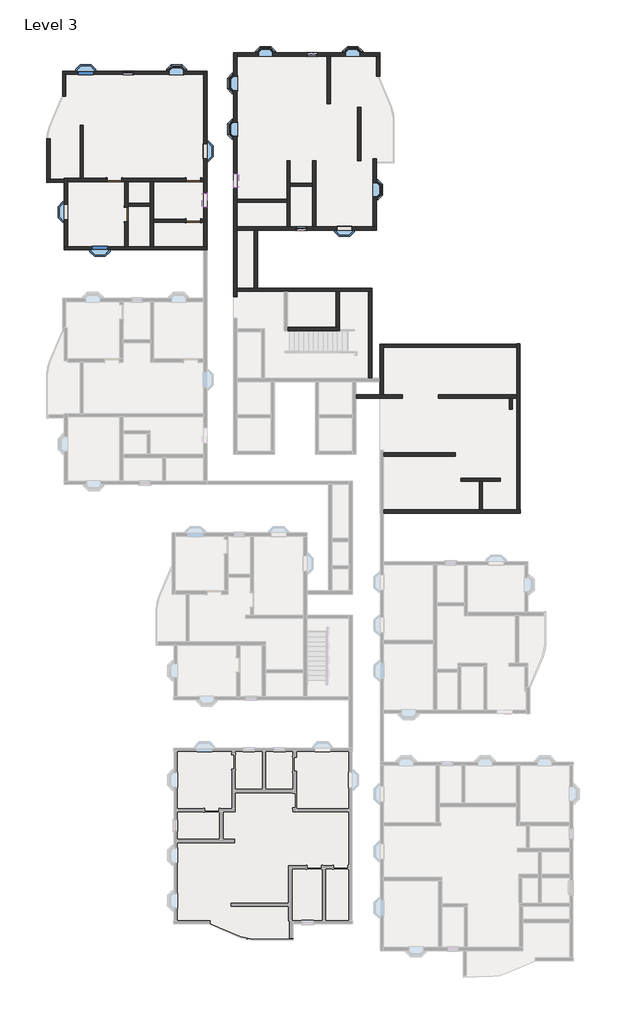
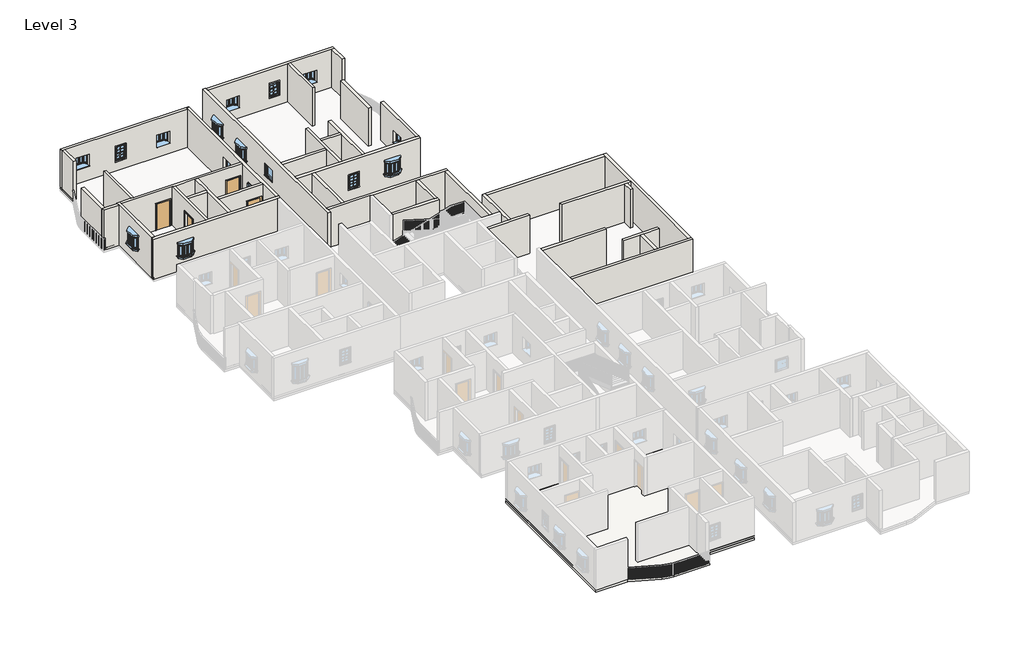
# One storey, part 4 of 14: 39 walls, 16 windows, 4 doors, 1 roof, 1 slab.
"""IFC4 building model written with IfcOpenShell, lengths in millimetres."""

from ifc_helpers import new_model, si_unit, point, frame, frame_2d, origin, place, context, project, spatial, polyline, circle_curve, trimmed, segment, composite_curve, outline, extrude, faceted_brep, transform, mapped, element, save
from components import door_719f80de, window_910x910mm_67ef725a, window_8debb0fa, windows_sgl_w_glazing_bars_910x910mm_256712d0

model = new_model("IFC4")

# Units and contexts
model_context = context("Model", 3, world=origin())
ifc_project = project(units=[si_unit("LENGTHUNIT", "METRE", prefix="MILLI")], contexts=[model_context])

# Site, building, storey
site = spatial("IfcSite", under=ifc_project)
building = spatial("IfcBuilding", under=site)
storey = spatial("IfcBuildingStorey", under=building, Name="Level 3", Elevation=6096.0)

# Doors
placement = place(None, origin())
door_shape = door_719f80de(model_context)
element("IfcDoor", 1, ObjectType="Single-Flush : 36\" x 84\"", at=placement, inside=storey, context=model_context, shape_type="MappedRepresentation", body=[
    mapped(door_shape, transform((-16068.1391351, 22048.4083494, 6096.0), x_axis=(1.0, 0.0, 0.0), y_axis=(0.0, 1.0, 0.0), z_axis=(0.0, 0.0, 1.0))),
])
element("IfcDoor", 2, ObjectType="Single-Flush : 36\" x 84\"", at=placement, inside=storey, context=model_context, shape_type="MappedRepresentation", body=[
    mapped(door_shape, transform((-15306.1391351, 19864.0083494, 6096.0), x_axis=(0.0, 1.0, 0.0), y_axis=(-1.0, 0.0, 0.0), z_axis=(0.0, 0.0, 1.0))),
])
element("IfcDoor", 3, ObjectType="Single-Flush : 36\" x 84\"", at=placement, inside=storey, context=model_context, shape_type="MappedRepresentation", body=[
    mapped(door_shape, transform((-11057.9891351, 19470.3083494, 6096.0), x_axis=(1.0, 0.0, 0.0), y_axis=(0.0, 1.0, 0.0), z_axis=(0.0, 0.0, 1.0))),
])
element("IfcDoor", 4, ObjectType="Single-Flush : 36\" x 84\"", at=placement, inside=storey, context=model_context, shape_type="MappedRepresentation", body=[
    mapped(door_shape, transform((-11057.9891351, 22048.4083494, 6096.0), x_axis=(1.0, 0.0, 0.0), y_axis=(0.0, 1.0, 0.0), z_axis=(0.0, 0.0, 1.0))),
])

# Roof
element("IfcRoof", 5, ObjectType="Generic - 12\"", at=placement, inside=storey, context=model_context, shape_type="SweptSolid", body=[
    extrude(outline(composite_curve([segment(polyline([(-10024.8708389, -25100.3416506), (-12290.487215, -25100.3416506), (-12290.487215, -13962.4416506), (-986.8891351, -13962.4416506), (-986.8891351, -25100.3416506), (-4746.0891351, -25100.3416506), (-4746.0891351, -26090.9416506), (-7315.6413127, -26090.9416506)]), True, "CONTINUOUS"), segment(trimmed(circle_curve(frame_2d((-7315.6413127, -24160.5416506)), 1930.4), [point((-7315.6413127, -26090.9416506))], [point((-8075.5356374, -25935.0851906))], False, "CARTESIAN"), True, "CONTINUOUS"), segment(polyline([(-8075.5356374, -25935.0851906), (-10024.8708389, -25100.3416506)]), True, "CONTINUOUS")], self_intersect=False)), frame((0.0, 0.0, 6096.0), z_axis=(0.0, 0.0, 1.0), x_axis=(1.0, 0.0, 0.0)), (0.0, 0.0, 1.0), 152.4),
])

# Slab
element("IfcSlab", 6, ObjectType="Generic - 12\"", at=placement, inside=storey, context=model_context, shape_type="SweptSolid", body=[
    extrude(outline(composite_curve([segment(polyline([(-10024.8708389, -25100.3416506), (-12290.487215, -25100.3416506), (-12290.487215, -13962.4416506), (-986.8891351, -13962.4416506), (-986.8891351, -25100.3416506), (-4746.0891351, -25100.3416506), (-4746.0891351, -26090.9416506), (-7315.6413127, -26090.9416506)]), True, "CONTINUOUS"), segment(trimmed(circle_curve(frame_2d((-7315.6413127, -24160.5416506)), 1930.4), [point((-7315.6413127, -26090.9416506))], [point((-8075.5356374, -25935.0851906))], False, "CARTESIAN"), True, "CONTINUOUS"), segment(polyline([(-8075.5356374, -25935.0851906), (-10024.8708389, -25100.3416506)]), True, "CONTINUOUS")], self_intersect=False)), frame((0.0, 0.0, 5943.6), z_axis=(0.0, 0.0, 1.0), x_axis=(1.0, 0.0, 0.0)), (0.0, 0.0, 1.0), 152.4),
])

# Walls
element("IfcWall", 7, ObjectType="4.5\" p", at=placement, inside=storey, context=model_context, shape_type="Brep", body=[
    faceted_brep([(-10600.7891351, 21946.8083494, 8229.6), (-10600.7891351, 21946.8083494, 6096.0), (-10397.5891351, 21946.8083494, 6096.0), (-10397.5891351, 21946.8083494, 9144.0), (-13578.9391351, 21946.8083494, 9144.0), (-13782.1391351, 21946.8083494, 9144.0), (-15204.5391351, 21946.8083494, 9144.0), (-15407.7391351, 21946.8083494, 9144.0), (-19033.5891351, 21946.8083494, 9144.0), (-19033.5891351, 21946.8083494, 6096.0), (-16525.3391351, 21946.8083494, 6096.0), (-16525.3391351, 21946.8083494, 8229.6), (-15610.9391351, 21946.8083494, 8229.6), (-15610.9391351, 21946.8083494, 6096.0), (-15407.7391351, 21946.8083494, 6096.0), (-15204.5391351, 21946.8083494, 6096.0), (-13782.1391351, 21946.8083494, 6096.0), (-13578.9391351, 21946.8083494, 6096.0), (-11515.1891351, 21946.8083494, 6096.0), (-11515.1891351, 21946.8083494, 8229.6), (-10397.5891351, 22150.0083494, 6096.0), (-10600.7891351, 22150.0083494, 6096.0), (-10600.7891351, 22150.0083494, 8229.6), (-11515.1891351, 22150.0083494, 8229.6), (-11515.1891351, 22150.0083494, 6096.0), (-15610.9391351, 22150.0083494, 6096.0), (-15610.9391351, 22150.0083494, 8229.6), (-16525.3391351, 22150.0083494, 8229.6), (-16525.3391351, 22150.0083494, 6096.0), (-18042.9891351, 22150.0083494, 6096.0), (-18246.1891351, 22150.0083494, 6096.0), (-19033.5891351, 22150.0083494, 6096.0), (-19033.5891351, 22150.0083494, 9144.0), (-18246.1891351, 22150.0083494, 9144.0), (-18042.9891351, 22150.0083494, 9144.0), (-10397.5891351, 22150.0083494, 9144.0)], [[[0, 1, 2, 3, 4, 5, 6, 7, 8, 9, 10, 11, 12, 13, 14, 15, 16, 17, 18, 19]], [[20, 21, 22, 23, 24, 25, 26, 27, 28, 29, 30, 31, 32, 33, 34, 35]], [[10, 9, 31, 30, 29, 28]], [[2, 1, 21, 20]], [[18, 17, 16, 15, 14, 13, 25, 24]], [[8, 7, 6, 5, 4, 3, 35, 34, 33, 32]], [[9, 8, 32, 31]], [[3, 2, 20, 35]], [[26, 25, 13, 12]], [[27, 26, 12, 11]], [[28, 27, 11, 10]], [[22, 21, 1, 0]], [[23, 22, 0, 19]], [[24, 23, 19, 18]]]),
])
element("IfcWall", 8, ObjectType="4.5\" p", at=placement, inside=storey, context=model_context, shape_type="Brep", body=[
    faceted_brep([(-15407.7391351, 21946.8083494, 6096.0), (-15407.7391351, 20321.2083494, 6096.0), (-15407.7391351, 20321.2083494, 8229.6), (-15407.7391351, 19406.8083494, 8229.6), (-15407.7391351, 19406.8083494, 6096.0), (-15407.7391351, 17812.9583494, 6096.0), (-15407.7391351, 17812.9583494, 9144.0), (-15407.7391351, 21946.8083494, 9144.0), (-15204.5391351, 20321.2083494, 8229.6), (-15204.5391351, 20321.2083494, 6096.0), (-15204.5391351, 20372.0083494, 6096.0), (-15204.5391351, 20575.2083494, 6096.0), (-15204.5391351, 21946.8083494, 6096.0), (-15204.5391351, 21946.8083494, 9144.0), (-15204.5391351, 20575.2083494, 9144.0), (-15204.5391351, 20372.0083494, 9144.0), (-15204.5391351, 17812.9583494, 9144.0), (-15204.5391351, 17812.9583494, 6096.0), (-15204.5391351, 19406.8083494, 6096.0), (-15204.5391351, 19406.8083494, 8229.6)], [[[0, 1, 2, 3, 4, 5, 6, 7]], [[8, 9, 10, 11, 12, 13, 14, 15, 16, 17, 18, 19]], [[18, 17, 5, 4]], [[12, 11, 10, 9, 1, 0]], [[7, 6, 16, 15, 14, 13]], [[6, 5, 17, 16]], [[0, 7, 13, 12]], [[2, 1, 9, 8]], [[3, 2, 8, 19]], [[4, 3, 19, 18]]]),
])
element("IfcWall", 9, ObjectType="4.5\" p", at=placement, inside=storey, context=model_context, shape_type="Brep", body=[
    faceted_brep([(-13782.1391351, 21946.8083494, 6096.0), (-13782.1391351, 20575.2083494, 6096.0), (-13782.1391351, 20372.0083494, 6096.0), (-13782.1391351, 17812.9583494, 6096.0), (-13782.1391351, 17812.9583494, 9144.0), (-13782.1391351, 20372.0083494, 9144.0), (-13782.1391351, 20575.2083494, 9144.0), (-13782.1391351, 21946.8083494, 9144.0), (-13578.9391351, 21946.8083494, 6096.0), (-13578.9391351, 21946.8083494, 9144.0), (-13578.9391351, 19571.9083494, 9144.0), (-13578.9391351, 19368.7083494, 9144.0), (-13578.9391351, 17812.9583494, 9144.0), (-13578.9391351, 17812.9583494, 6096.0), (-13578.9391351, 19368.7083494, 6096.0), (-13578.9391351, 19571.9083494, 6096.0)], [[[0, 1, 2, 3, 4, 5, 6, 7]], [[8, 9, 10, 11, 12, 13, 14, 15]], [[3, 2, 1, 0, 8, 15, 14, 13]], [[7, 6, 5, 4, 12, 11, 10, 9]], [[4, 3, 13, 12]], [[0, 7, 9, 8]]]),
])
element("IfcWall", 10, ObjectType="4.5\" p", at=placement, inside=storey, context=model_context, shape_type="SweptSolid", body=[
    extrude(outline(polyline([(-13782.1391351, 20372.0083494), (-15204.5391351, 20372.0083494), (-15204.5391351, 20575.2083494), (-13782.1391351, 20575.2083494), (-13782.1391351, 20372.0083494)])), frame((0.0, 0.0, 6096.0), z_axis=(0.0, 0.0, 1.0), x_axis=(1.0, 0.0, 0.0)), (0.0, 0.0, 1.0), 3048.0),
])
element("IfcWall", 11, ObjectType="4.5\" p", at=placement, inside=storey, context=model_context, shape_type="SweptSolid", body=[
    extrude(outline(polyline([(8229.6, -10600.7891351), (6096.0, -10600.7891351), (6096.0, -10397.5891351), (9144.0, -10397.5891351), (9144.0, -13578.9391351), (6096.0, -13578.9391351), (6096.0, -11515.1891351), (8229.6, -11515.1891351), (8229.6, -10600.7891351)])), frame((0.0, 19368.7083494, 0.0), z_axis=(0.0, 1.0, 0.0), x_axis=(0.0, 0.0, 1.0)), (0.0, 0.0, 1.0), 203.2),
])
element("IfcWall", 12, ObjectType="4.5\" p", at=placement, inside=storey, context=model_context, shape_type="SweptSolid", body=[
    extrude(outline(polyline([(-18246.1891351, 22150.0083494), (-18246.1891351, 25515.5083494), (-18042.9891351, 25515.5083494), (-18042.9891351, 22150.0083494), (-18246.1891351, 22150.0083494)])), frame((0.0, 0.0, 6096.0), z_axis=(0.0, 0.0, 1.0), x_axis=(1.0, 0.0, 0.0)), (0.0, 0.0, 1.0), 3048.0),
])
element("IfcWall", 13, ObjectType="4.5\" p", at=placement, inside=storey, context=model_context, shape_type="SweptSolid", body=[
    extrude(outline(polyline([(-6993.9891351, 18875.1215905), (-6993.9891351, 15192.1215905), (-7197.1891351, 15192.1215905), (-7197.1891351, 18875.1215905), (-6993.9891351, 18875.1215905)])), frame((0.0, 0.0, 6096.0), z_axis=(0.0, 0.0, 1.0), x_axis=(1.0, 0.0, 0.0)), (0.0, 0.0, 1.0), 3048.0),
])
element("IfcWall", 14, ObjectType="4.5\" p", at=placement, inside=storey, context=model_context, shape_type="Brep", body=[
    faceted_brep([(-8289.3891351, 18875.1215905, 6096.0), (-7197.1891351, 18875.1215905, 6096.0), (-6993.9891351, 18875.1215905, 6096.0), (562.5108649, 18875.1215905, 6096.0), (562.5108649, 18875.1215905, 9144.0), (-6993.9891351, 18875.1215905, 9144.0), (-7197.1891351, 18875.1215905, 9144.0), (-8289.3891351, 18875.1215905, 9144.0), (-1017.6641351, 18875.1215905, 8206.0), (-1017.6641351, 18875.1215905, 7296.0), (-1927.6641351, 18875.1215905, 7296.0), (-1927.6641351, 18875.1215905, 8206.0), (-3876.1391351, 18875.1215905, 8077.2), (-3876.1391351, 18875.1215905, 7010.4), (-4536.5391351, 18875.1215905, 7010.4), (-4536.5391351, 18875.1215905, 8077.2), (-8289.3891351, 19078.3215905, 6096.0), (-8289.3891351, 19078.3215905, 9144.0), (-5120.7391351, 19078.3215905, 9144.0), (-4917.5391351, 19078.3215905, 9144.0), (-3495.1391351, 19078.3215905, 9144.0), (-3291.9391351, 19078.3215905, 9144.0), (346.6108649, 19078.3215905, 9144.0), (549.8108649, 19078.3215905, 9144.0), (562.5108649, 19078.3215905, 9144.0), (562.5108649, 19078.3215905, 6096.0), (549.8108649, 19078.3215905, 6096.0), (346.6108649, 19078.3215905, 6096.0), (-3291.9391351, 19078.3215905, 6096.0), (-3495.1391351, 19078.3215905, 6096.0), (-4917.5391351, 19078.3215905, 6096.0), (-5120.7391351, 19078.3215905, 6096.0), (-1017.6641351, 19078.3215905, 8206.0), (-1927.6641351, 19078.3215905, 8206.0), (-1927.6641351, 19078.3215905, 7296.0), (-1017.6641351, 19078.3215905, 7296.0), (-3876.1391351, 19078.3215905, 8077.2), (-4536.5391351, 19078.3215905, 8077.2), (-4536.5391351, 19078.3215905, 7010.4), (-3876.1391351, 19078.3215905, 7010.4)], [[[0, 1, 2, 3, 4, 5, 6, 7], [8, 9, 10, 11], [12, 13, 14, 15]], [[16, 17, 18, 19, 20, 21, 22, 23, 24, 25, 26, 27, 28, 29, 30, 31], [32, 33, 34, 35], [36, 37, 38, 39]], [[3, 2, 1, 0, 16, 31, 30, 29, 28, 27, 26, 25]], [[4, 3, 25, 24]], [[7, 6, 5, 4, 24, 23, 22, 21, 20, 19, 18, 17]], [[0, 7, 17, 16]], [[9, 8, 32, 35]], [[10, 9, 35, 34]], [[11, 10, 34, 33]], [[8, 11, 33, 32]], [[13, 12, 36, 39]], [[14, 13, 39, 38]], [[15, 14, 38, 37]], [[12, 15, 37, 36]]]),
])
element("IfcWall", 15, ObjectType="4.5\" p", at=placement, inside=storey, context=model_context, shape_type="SweptSolid", body=[
    extrude(outline(polyline([(19078.3215905, 6096.0), (19078.3215905, 9144.0), (23396.3215905, 9144.0), (23396.3215905, 6096.0), (19078.3215905, 6096.0)]), holes=[polyline([(21882.8215905, 7920.4), (20972.8215905, 7920.4), (20972.8215905, 7010.4), (21882.8215905, 7010.4), (21882.8215905, 7920.4)])]), frame((346.6108649, 0.0, 0.0), z_axis=(1.0, 0.0, 0.0), x_axis=(0.0, 1.0, 0.0)), (0.0, 0.0, 1.0), 203.2),
])
element("IfcWall", 16, ObjectType="4.5\" p", at=placement, inside=storey, context=model_context, shape_type="SweptSolid", body=[
    extrude(outline(polyline([(-5120.7391351, 20634.0715905), (-8289.3891351, 20634.0715905), (-8289.3891351, 20837.2715905), (-5120.7391351, 20837.2715905), (-5120.7391351, 20634.0715905)])), frame((0.0, 0.0, 6096.0), z_axis=(0.0, 0.0, 1.0), x_axis=(1.0, 0.0, 0.0)), (0.0, 0.0, 1.0), 3048.0),
])
element("IfcWall", 17, ObjectType="4.5\" p", at=placement, inside=storey, context=model_context, shape_type="Brep", body=[
    faceted_brep([(-5120.7391351, 23256.6215905, 6096.0), (-5120.7391351, 20837.2715905, 6096.0), (-5120.7391351, 20634.0715905, 6096.0), (-5120.7391351, 19078.3215905, 6096.0), (-5120.7391351, 19078.3215905, 9144.0), (-5120.7391351, 20634.0715905, 9144.0), (-5120.7391351, 20837.2715905, 9144.0), (-5120.7391351, 23256.6215905, 9144.0), (-4917.5391351, 23256.6215905, 6096.0), (-4917.5391351, 23256.6215905, 9144.0), (-4917.5391351, 21853.2715905, 9144.0), (-4917.5391351, 21650.0715905, 9144.0), (-4917.5391351, 19078.3215905, 9144.0), (-4917.5391351, 19078.3215905, 6096.0), (-4917.5391351, 21650.0715905, 6096.0), (-4917.5391351, 21853.2715905, 6096.0)], [[[0, 1, 2, 3, 4, 5, 6, 7]], [[8, 9, 10, 11, 12, 13, 14, 15]], [[3, 2, 1, 0, 8, 15, 14, 13]], [[7, 6, 5, 4, 12, 11, 10, 9]], [[0, 7, 9, 8]], [[4, 3, 13, 12]]]),
])
element("IfcWall", 18, ObjectType="4.5\" p", at=placement, inside=storey, context=model_context, shape_type="Brep", body=[
    faceted_brep([(-3495.1391351, 23256.6215905, 6096.0), (-3495.1391351, 21853.2715905, 6096.0), (-3495.1391351, 21650.0715905, 6096.0), (-3495.1391351, 19078.3215905, 6096.0), (-3495.1391351, 19078.3215905, 9144.0), (-3495.1391351, 21650.0715905, 9144.0), (-3495.1391351, 21853.2715905, 9144.0), (-3495.1391351, 23256.6215905, 9144.0), (-3291.9391351, 23256.6215905, 6096.0), (-3291.9391351, 23256.6215905, 9144.0), (-3291.9391351, 19078.3215905, 9144.0), (-3291.9391351, 19078.3215905, 6096.0)], [[[0, 1, 2, 3, 4, 5, 6, 7]], [[8, 9, 10, 11]], [[3, 2, 1, 0, 8, 11]], [[7, 6, 5, 4, 10, 9]], [[0, 7, 9, 8]], [[4, 3, 11, 10]]]),
])
element("IfcWall", 19, ObjectType="4.5\" p", at=placement, inside=storey, context=model_context, shape_type="SweptSolid", body=[
    extrude(outline(polyline([(-3495.1391351, 21650.0715905), (-4917.5391351, 21650.0715905), (-4917.5391351, 21853.2715905), (-3495.1391351, 21853.2715905), (-3495.1391351, 21650.0715905)])), frame((0.0, 0.0, 6096.0), z_axis=(0.0, 0.0, 1.0), x_axis=(1.0, 0.0, 0.0)), (0.0, 0.0, 1.0), 3048.0),
])
element("IfcWall", 20, ObjectType="4.5\" p", at=placement, inside=storey, context=model_context, shape_type="SweptSolid", body=[
    extrude(outline(polyline([(-1799.6891351, 14988.9215905), (-1799.6891351, 12709.2715905), (-2002.8891351, 12709.2715905), (-2002.8891351, 14988.9215905), (-1799.6891351, 14988.9215905)])), frame((0.0, 0.0, 6096.0), z_axis=(0.0, 0.0, 1.0), x_axis=(1.0, 0.0, 0.0)), (0.0, 0.0, 1.0), 3048.0),
])
element("IfcWall", 21, ObjectType="4.5\" p", at=placement, inside=storey, context=model_context, shape_type="Brep", body=[
    faceted_brep([(-5095.3391351, 12506.0715905, 6096.0), (-1786.9891351, 12506.0715905, 6096.0), (-1786.9891351, 12506.0715905, 9144.0), (-5095.3391351, 12506.0715905, 9144.0), (-5095.3391351, 12709.2715905, 6096.0), (-5095.3391351, 12709.2715905, 9144.0), (-2002.8891351, 12709.2715905, 9144.0), (-1799.6891351, 12709.2715905, 9144.0), (-1786.9891351, 12709.2715905, 9144.0), (-1786.9891351, 12709.2715905, 6096.0), (-1799.6891351, 12709.2715905, 6096.0), (-2002.8891351, 12709.2715905, 6096.0)], [[[0, 1, 2, 3]], [[4, 5, 6, 7, 8, 9, 10, 11]], [[1, 0, 4, 11, 10, 9]], [[2, 1, 9, 8]], [[3, 2, 8, 7, 6, 5]], [[0, 3, 5, 4]]]),
])
element("IfcWall", 22, ObjectType="4.5\" p", at=placement, inside=storey, context=model_context, shape_type="Brep", body=[
    faceted_brep([(-745.5891351, 8223.6457306, 6096.0), (2209.4205024, 8223.6457306, 6096.0), (2209.4205024, 8223.6457306, 9144.0), (-745.5891351, 8223.6457306, 9144.0), (-745.5891351, 8426.8457306, 6096.0), (-745.5891351, 8426.8457306, 9144.0), (793.5880523, 8426.8457306, 9144.0), (996.7880523, 8426.8457306, 9144.0), (2209.4205024, 8426.8457306, 9144.0), (2209.4205024, 8426.8457306, 6096.0), (996.7880523, 8426.8457306, 6096.0), (793.5880523, 8426.8457306, 6096.0)], [[[0, 1, 2, 3]], [[4, 5, 6, 7, 8, 9, 10, 11]], [[1, 0, 4, 11, 10, 9]], [[2, 1, 9, 8]], [[3, 2, 8, 7, 6, 5]], [[0, 3, 5, 4]]]),
])
element("IfcWall", 23, ObjectType="4.5\" p", at=placement, inside=storey, context=model_context, shape_type="Brep", body=[
    faceted_brep([(996.7880523, 8426.8457306, 6096.0), (996.7880523, 11443.0957306, 6096.0), (996.7880523, 11646.2957306, 6096.0), (996.7880523, 11646.2957306, 9144.0), (996.7880523, 11443.0957306, 9144.0), (996.7880523, 8426.8457306, 9144.0), (793.5880523, 8426.8457306, 6096.0), (793.5880523, 8426.8457306, 9144.0), (793.5880523, 9275.2949943, 9144.0), (793.5880523, 9478.4949943, 9144.0), (793.5880523, 11646.2957306, 9144.0), (793.5880523, 11646.2957306, 6096.0), (793.5880523, 9478.4949943, 6096.0), (793.5880523, 9275.2949943, 6096.0)], [[[0, 1, 2, 3, 4, 5]], [[6, 7, 8, 9, 10, 11, 12, 13]], [[2, 1, 0, 6, 13, 12, 11]], [[5, 4, 3, 10, 9, 8, 7]], [[0, 5, 7, 6]], [[3, 2, 11, 10]]]),
])
element("IfcWall", 24, ObjectType="4.5\" p", at=placement, inside=storey, context=model_context, shape_type="Brep", body=[
    faceted_brep([(9461.3380523, 8426.8457306, 6096.0), (4492.3034266, 8426.8457306, 6096.0), (4492.3034266, 8426.8457306, 9144.0), (9461.3380523, 8426.8457306, 9144.0), (9461.3380523, 8223.6457306, 6096.0), (9461.3380523, 8223.6457306, 9144.0), (9181.9380523, 8223.6457306, 9144.0), (8978.7380523, 8223.6457306, 9144.0), (4492.3034266, 8223.6457306, 9144.0), (4492.3034266, 8223.6457306, 6096.0), (8978.7380523, 8223.6457306, 6096.0), (9181.9380523, 8223.6457306, 6096.0)], [[[0, 1, 2, 3]], [[4, 5, 6, 7, 8, 9, 10, 11]], [[1, 0, 4, 11, 10, 9]], [[2, 1, 9, 8]], [[3, 2, 8, 7, 6, 5]], [[0, 3, 5, 4]]]),
])
element("IfcWall", 25, ObjectType="4.5\" p", at=placement, inside=storey, context=model_context, shape_type="Brep", body=[
    faceted_brep([(1007.0108649, 940.1957306, 6096.0), (9677.2380523, 940.1957306, 6096.0), (9677.2380523, 940.1957306, 9144.0), (1007.0108649, 940.1957306, 9144.0), (1007.0108649, 1143.3957306, 6096.0), (1007.0108649, 1143.3957306, 9144.0), (7073.7380523, 1143.3957306, 9144.0), (7276.9380523, 1143.3957306, 9144.0), (9461.3380523, 1143.3957306, 9144.0), (9664.5380523, 1143.3957306, 9144.0), (9677.2380523, 1143.3957306, 9144.0), (9677.2380523, 1143.3957306, 6096.0), (9664.5380523, 1143.3957306, 6096.0), (9461.3380523, 1143.3957306, 6096.0), (7276.9380523, 1143.3957306, 6096.0), (7073.7380523, 1143.3957306, 6096.0)], [[[0, 1, 2, 3]], [[4, 5, 6, 7, 8, 9, 10, 11, 12, 13, 14, 15]], [[1, 0, 4, 15, 14, 13, 12, 11]], [[2, 1, 11, 10]], [[3, 2, 10, 9, 8, 7, 6, 5]], [[0, 3, 5, 4]]]),
])
element("IfcWall", 26, ObjectType="4.5\" p", at=placement, inside=storey, context=model_context, shape_type="Brep", body=[
    faceted_brep([(9664.5380523, 1143.3957306, 6096.0), (9664.5380523, 11658.9957306, 6096.0), (9664.5380523, 11658.9957306, 9144.0), (9664.5380523, 1143.3957306, 9144.0), (9461.3380523, 1143.3957306, 6096.0), (9461.3380523, 1143.3957306, 9144.0), (9461.3380523, 8223.6457306, 9144.0), (9461.3380523, 8426.8457306, 9144.0), (9461.3380523, 11443.0957306, 9144.0), (9461.3380523, 11646.2957306, 9144.0), (9461.3380523, 11658.9957306, 9144.0), (9461.3380523, 11658.9957306, 6096.0), (9461.3380523, 11646.2957306, 6096.0), (9461.3380523, 11443.0957306, 6096.0), (9461.3380523, 8426.8457306, 6096.0), (9461.3380523, 8223.6457306, 6096.0)], [[[0, 1, 2, 3]], [[4, 5, 6, 7, 8, 9, 10, 11, 12, 13, 14, 15]], [[1, 0, 4, 15, 14, 13, 12, 11]], [[2, 1, 11, 10]], [[3, 2, 10, 9, 8, 7, 6, 5]], [[0, 3, 5, 4]]]),
])
element("IfcWall", 27, ObjectType="4.5\" p", at=placement, inside=storey, context=model_context, shape_type="SweptSolid", body=[
    extrude(outline(polyline([(-643.9891351, 23256.6215905), (-643.9891351, 26659.3286213), (-440.7891351, 26659.3286213), (-440.7891351, 23256.6215905), (-643.9891351, 23256.6215905)])), frame((0.0, 0.0, 6096.0), z_axis=(0.0, 0.0, 1.0), x_axis=(1.0, 0.0, 0.0)), (0.0, 0.0, 1.0), 3048.0),
])
element("IfcWall", 28, ObjectType="4.5\" p", at=placement, inside=storey, context=model_context, shape_type="SweptSolid", body=[
    extrude(outline(polyline([(-2568.0391351, 26862.5286213), (-2568.0391351, 29898.7215905), (-2364.8391351, 29898.7215905), (-2364.8391351, 26862.5286213), (-2568.0391351, 26862.5286213)])), frame((0.0, 0.0, 6096.0), z_axis=(0.0, 0.0, 1.0), x_axis=(1.0, 0.0, 0.0)), (0.0, 0.0, 1.0), 3048.0),
])
element("IfcWall", 29, ObjectType="4.5\" p", at=placement, inside=storey, context=model_context, shape_type="SweptSolid", body=[
    extrude(outline(polyline([(765.7108649, 29898.7215905), (765.7108649, 28631.1875845), (562.5108649, 28631.1875845), (562.5108649, 29898.7215905), (765.7108649, 29898.7215905)])), frame((0.0, 0.0, 6096.0), z_axis=(0.0, 0.0, 1.0), x_axis=(1.0, 0.0, 0.0)), (0.0, 0.0, 1.0), 3048.0),
])
element("IfcWall", 30, ObjectType="9\" w", at=placement, inside=storey, context=model_context, shape_type="Brep", body=[
    faceted_brep([(-10181.6891351, 17812.9583494, 6096.0), (-10194.3891351, 17812.9583494, 6096.0), (-10397.5891351, 17812.9583494, 6096.0), (-13578.9391351, 17812.9583494, 6096.0), (-13782.1391351, 17812.9583494, 6096.0), (-15204.5391351, 17812.9583494, 6096.0), (-15407.7391351, 17812.9583494, 6096.0), (-19033.5891351, 17812.9583494, 6096.0), (-19236.7891351, 17812.9583494, 6096.0), (-19249.4891351, 17812.9583494, 6096.0), (-19249.4891351, 17812.9583494, 9144.0), (-19236.7891351, 17812.9583494, 9144.0), (-19033.5891351, 17812.9583494, 9144.0), (-15407.7391351, 17812.9583494, 9144.0), (-15204.5391351, 17812.9583494, 9144.0), (-13782.1391351, 17812.9583494, 9144.0), (-13578.9391351, 17812.9583494, 9144.0), (-10397.5891351, 17812.9583494, 9144.0), (-10194.3891351, 17812.9583494, 9144.0), (-10181.6891351, 17812.9583494, 9144.0), (-16527.5391351, 17812.9583494, 8206.0), (-17437.5391351, 17812.9583494, 8206.0), (-17437.5391351, 17812.9583494, 7296.0), (-16527.5391351, 17812.9583494, 7296.0), (-10181.6891351, 17609.7583494, 6096.0), (-10181.6891351, 17609.7583494, 9144.0), (-19249.4891351, 17609.7583494, 9144.0), (-19249.4891351, 17609.7583494, 6096.0), (-16527.5391351, 17609.7583494, 8206.0), (-16527.5391351, 17609.7583494, 7296.0), (-17437.5391351, 17609.7583494, 7296.0), (-17437.5391351, 17609.7583494, 8206.0)], [[[0, 1, 2, 3, 4, 5, 6, 7, 8, 9, 10, 11, 12, 13, 14, 15, 16, 17, 18, 19], [20, 21, 22, 23]], [[24, 25, 26, 27], [28, 29, 30, 31]], [[9, 8, 7, 6, 5, 4, 3, 2, 1, 0, 24, 27]], [[10, 9, 27, 26]], [[19, 18, 17, 16, 15, 14, 13, 12, 11, 10, 26, 25]], [[0, 19, 25, 24]], [[29, 28, 20, 23]], [[30, 29, 23, 22]], [[31, 30, 22, 21]], [[28, 31, 21, 20]]]),
])
element("IfcWall", 31, ObjectType="9\" w", at=placement, inside=storey, context=model_context, shape_type="Brep", body=[
    faceted_brep([(-19033.5891351, 17812.9583494, 6096.0), (-19033.5891351, 21946.8083494, 6096.0), (-19033.5891351, 22150.0083494, 6096.0), (-19033.5891351, 22150.0083494, 9144.0), (-19033.5891351, 21946.8083494, 9144.0), (-19033.5891351, 17812.9583494, 9144.0), (-19033.5891351, 19555.0583494, 8206.0), (-19033.5891351, 20465.0583494, 8206.0), (-19033.5891351, 20465.0583494, 7296.0), (-19033.5891351, 19555.0583494, 7296.0), (-19236.7891351, 17812.9583494, 6096.0), (-19236.7891351, 17812.9583494, 9144.0), (-19236.7891351, 21889.6583494, 9144.0), (-19236.7891351, 22092.8583494, 9144.0), (-19236.7891351, 22150.0083494, 9144.0), (-19236.7891351, 22150.0083494, 6096.0), (-19236.7891351, 22092.8583494, 6096.0), (-19236.7891351, 21889.6583494, 6096.0), (-19236.7891351, 19555.0583494, 8206.0), (-19236.7891351, 19555.0583494, 7296.0), (-19236.7891351, 20465.0583494, 7296.0), (-19236.7891351, 20465.0583494, 8206.0)], [[[0, 1, 2, 3, 4, 5], [6, 7, 8, 9]], [[10, 11, 12, 13, 14, 15, 16, 17], [18, 19, 20, 21]], [[2, 1, 0, 10, 17, 16, 15]], [[5, 4, 3, 14, 13, 12, 11]], [[0, 5, 11, 10]], [[3, 2, 15, 14]], [[19, 18, 6, 9]], [[20, 19, 9, 8]], [[21, 20, 8, 7]], [[18, 21, 7, 6]]]),
])
element("IfcWall", 32, ObjectType="9\" w", at=placement, inside=storey, context=model_context, shape_type="Brep", body=[
    faceted_brep([(-10194.3891351, 17812.9583494, 6096.0), (-10194.3891351, 28849.2583494, 6096.0), (-10194.3891351, 28849.2583494, 9144.0), (-10194.3891351, 17812.9583494, 9144.0), (-10194.3891351, 24319.5083494, 8206.0), (-10194.3891351, 24319.5083494, 7296.0), (-10194.3891351, 23409.5083494, 7296.0), (-10194.3891351, 23409.5083494, 8206.0), (-10194.3891351, 20304.3583494, 8206.0), (-10194.3891351, 21214.3583494, 8206.0), (-10194.3891351, 21214.3583494, 7296.0), (-10194.3891351, 20304.3583494, 7296.0), (-10397.5891351, 17812.9583494, 6096.0), (-10397.5891351, 17812.9583494, 9144.0), (-10397.5891351, 19368.7083494, 9144.0), (-10397.5891351, 19571.9083494, 9144.0), (-10397.5891351, 21946.8083494, 9144.0), (-10397.5891351, 22150.0083494, 9144.0), (-10397.5891351, 28849.2583494, 9144.0), (-10397.5891351, 28849.2583494, 6096.0), (-10397.5891351, 22150.0083494, 6096.0), (-10397.5891351, 21946.8083494, 6096.0), (-10397.5891351, 19571.9083494, 6096.0), (-10397.5891351, 19368.7083494, 6096.0), (-10397.5891351, 24319.5083494, 8206.0), (-10397.5891351, 23409.5083494, 8206.0), (-10397.5891351, 23409.5083494, 7296.0), (-10397.5891351, 24319.5083494, 7296.0), (-10397.5891351, 20304.3583494, 8206.0), (-10397.5891351, 20304.3583494, 7296.0), (-10397.5891351, 21214.3583494, 7296.0), (-10397.5891351, 21214.3583494, 8206.0)], [[[0, 1, 2, 3], [4, 5, 6, 7], [8, 9, 10, 11]], [[12, 13, 14, 15, 16, 17, 18, 19, 20, 21, 22, 23], [24, 25, 26, 27], [28, 29, 30, 31]], [[1, 0, 12, 23, 22, 21, 20, 19]], [[2, 1, 19, 18]], [[3, 2, 18, 17, 16, 15, 14, 13]], [[0, 3, 13, 12]], [[5, 4, 24, 27]], [[6, 5, 27, 26]], [[7, 6, 26, 25]], [[4, 7, 25, 24]], [[29, 28, 8, 11]], [[30, 29, 11, 10]], [[31, 30, 10, 9]], [[28, 31, 9, 8]]]),
])
element("IfcWall", 33, ObjectType="9\" w", at=placement, inside=storey, context=model_context, shape_type="Brep", body=[
    faceted_brep([(-20341.6891351, 21889.6583494, 6096.0), (-19236.7891351, 21889.6583494, 6096.0), (-19236.7891351, 21889.6583494, 9144.0), (-20341.6891351, 21889.6583494, 9144.0), (-20341.6891351, 22092.8583494, 6096.0), (-20341.6891351, 22092.8583494, 9144.0), (-20138.4891351, 22092.8583494, 9144.0), (-19236.7891351, 22092.8583494, 9144.0), (-19236.7891351, 22092.8583494, 6096.0), (-20138.4891351, 22092.8583494, 6096.0)], [[[0, 1, 2, 3]], [[4, 5, 6, 7, 8, 9]], [[1, 0, 4, 9, 8]], [[3, 2, 7, 6, 5]], [[0, 3, 5, 4]], [[2, 1, 8, 7]]]),
])
element("IfcWall", 34, ObjectType="9\" w", at=placement, inside=storey, context=model_context, shape_type="SweptSolid", body=[
    extrude(outline(polyline([(-20341.6891351, 22092.8583494), (-20341.6891351, 24656.5948172), (-20138.4891351, 24656.5948172), (-20138.4891351, 22092.8583494), (-20341.6891351, 22092.8583494)])), frame((0.0, 0.0, 6096.0), z_axis=(0.0, 0.0, 1.0), x_axis=(1.0, 0.0, 0.0)), (0.0, 0.0, 1.0), 3048.0),
])
element("IfcWall", 35, ObjectType="9\" w", at=placement, inside=storey, context=model_context, shape_type="Brep", body=[
    faceted_brep([(-8492.5891351, 30114.6215905, 6096.0), (-8492.5891351, 14654.9471999, 6096.0), (-8492.5891351, 14654.9471999, 9144.0), (-8492.5891351, 30114.6215905, 9144.0), (-8492.5891351, 27703.9922564, 7920.4), (-8492.5891351, 27703.9922564, 7010.4), (-8492.5891351, 28613.9922564, 7010.4), (-8492.5891351, 28613.9922564, 7920.4), (-8492.5891351, 24808.3922564, 7920.4), (-8492.5891351, 24808.3922564, 7010.4), (-8492.5891351, 25718.3922564, 7010.4), (-8492.5891351, 25718.3922564, 7920.4), (-8492.5891351, 22451.1465905, 8206.0), (-8492.5891351, 21541.1465905, 8206.0), (-8492.5891351, 21541.1465905, 7296.0), (-8492.5891351, 22451.1465905, 7296.0), (-8289.3891351, 30114.6215905, 6096.0), (-8289.3891351, 30114.6215905, 9144.0), (-8289.3891351, 30101.9215905, 9144.0), (-8289.3891351, 29898.7215905, 9144.0), (-8289.3891351, 20837.2715905, 9144.0), (-8289.3891351, 20634.0715905, 9144.0), (-8289.3891351, 19078.3215905, 9144.0), (-8289.3891351, 18875.1215905, 9144.0), (-8289.3891351, 15192.1215905, 9144.0), (-8289.3891351, 14988.9215905, 9144.0), (-8289.3891351, 14654.9471999, 9144.0), (-8289.3891351, 14654.9471999, 6096.0), (-8289.3891351, 14988.9215905, 6096.0), (-8289.3891351, 15192.1215905, 6096.0), (-8289.3891351, 18875.1215905, 6096.0), (-8289.3891351, 19078.3215905, 6096.0), (-8289.3891351, 20634.0715905, 6096.0), (-8289.3891351, 20837.2715905, 6096.0), (-8289.3891351, 29898.7215905, 6096.0), (-8289.3891351, 30101.9215905, 6096.0), (-8289.3891351, 27703.9922564, 7920.4), (-8289.3891351, 28613.9922564, 7920.4), (-8289.3891351, 28613.9922564, 7010.4), (-8289.3891351, 27703.9922564, 7010.4), (-8289.3891351, 24808.3922564, 7920.4), (-8289.3891351, 25718.3922564, 7920.4), (-8289.3891351, 25718.3922564, 7010.4), (-8289.3891351, 24808.3922564, 7010.4), (-8289.3891351, 22451.1465905, 8206.0), (-8289.3891351, 22451.1465905, 7296.0), (-8289.3891351, 21541.1465905, 7296.0), (-8289.3891351, 21541.1465905, 8206.0)], [[[0, 1, 2, 3], [4, 5, 6, 7], [8, 9, 10, 11], [12, 13, 14, 15]], [[16, 17, 18, 19, 20, 21, 22, 23, 24, 25, 26, 27, 28, 29, 30, 31, 32, 33, 34, 35], [36, 37, 38, 39], [40, 41, 42, 43], [44, 45, 46, 47]], [[1, 0, 16, 35, 34, 33, 32, 31, 30, 29, 28, 27]], [[2, 1, 27, 26]], [[3, 2, 26, 25, 24, 23, 22, 21, 20, 19, 18, 17]], [[0, 3, 17, 16]], [[5, 4, 36, 39]], [[6, 5, 39, 38]], [[7, 6, 38, 37]], [[4, 7, 37, 36]], [[9, 8, 40, 43]], [[10, 9, 43, 42]], [[11, 10, 42, 41]], [[8, 11, 41, 40]], [[45, 44, 12, 15]], [[46, 45, 15, 14]], [[47, 46, 14, 13]], [[44, 47, 13, 12]]]),
])
element("IfcWall", 36, ObjectType="9\" w", at=placement, inside=storey, context=model_context, shape_type="Brep", body=[
    faceted_brep([(-8289.3891351, 14988.9215905, 6096.0), (-5298.5391351, 14988.9215905, 6096.0), (-5095.3391351, 14988.9215905, 6096.0), (-2002.8891351, 14988.9215905, 6096.0), (-1799.6891351, 14988.9215905, 6096.0), (54.5108649, 14988.9215905, 6096.0), (257.7108649, 14988.9215905, 6096.0), (270.4108649, 14988.9215905, 6096.0), (270.4108649, 14988.9215905, 9144.0), (257.7108649, 14988.9215905, 9144.0), (54.5108649, 14988.9215905, 9144.0), (-1799.6891351, 14988.9215905, 9144.0), (-2002.8891351, 14988.9215905, 9144.0), (-5095.3391351, 14988.9215905, 9144.0), (-5298.5391351, 14988.9215905, 9144.0), (-8289.3891351, 14988.9215905, 9144.0), (-8289.3891351, 15192.1215905, 6096.0), (-8289.3891351, 15192.1215905, 9144.0), (-7197.1891351, 15192.1215905, 9144.0), (-6993.9891351, 15192.1215905, 9144.0), (270.4108649, 15192.1215905, 9144.0), (270.4108649, 15192.1215905, 6096.0), (-6993.9891351, 15192.1215905, 6096.0), (-7197.1891351, 15192.1215905, 6096.0)], [[[0, 1, 2, 3, 4, 5, 6, 7, 8, 9, 10, 11, 12, 13, 14, 15]], [[16, 17, 18, 19, 20, 21, 22, 23]], [[7, 6, 5, 4, 3, 2, 1, 0, 16, 23, 22, 21]], [[8, 7, 21, 20]], [[15, 14, 13, 12, 11, 10, 9, 8, 20, 19, 18, 17]], [[0, 15, 17, 16]]]),
])
element("IfcWall", 37, ObjectType="9\" w", at=placement, inside=storey, context=model_context, shape_type="SweptSolid", body=[
    extrude(outline(polyline([(54.5108649, 9478.4949943), (54.5108649, 14988.9215905), (257.7108649, 14988.9215905), (257.7108649, 9478.4949943), (54.5108649, 9478.4949943)])), frame((0.0, 0.0, 6096.0), z_axis=(0.0, 0.0, 1.0), x_axis=(1.0, 0.0, 0.0)), (0.0, 0.0, 1.0), 3048.0),
])
element("IfcWall", 38, ObjectType="9\" w", at=placement, inside=storey, context=model_context, shape_type="SweptSolid", body=[
    extrude(outline(polyline([(9461.3380523, 11443.0957306), (996.7880523, 11443.0957306), (996.7880523, 11646.2957306), (9461.3380523, 11646.2957306), (9461.3380523, 11443.0957306)])), frame((0.0, 0.0, 6096.0), z_axis=(0.0, 0.0, 1.0), x_axis=(1.0, 0.0, 0.0)), (0.0, 0.0, 1.0), 3048.0),
])
element("IfcWall", 39, ObjectType="9\" w", at=placement, inside=storey, context=model_context, shape_type="SweptSolid", body=[
    extrude(outline(polyline([(8978.7380523, 7506.0957306), (8978.7380523, 8223.6457306), (9181.9380523, 8223.6457306), (9181.9380523, 7506.0957306), (8978.7380523, 7506.0957306)])), frame((0.0, 0.0, 6096.0), z_axis=(0.0, 0.0, 1.0), x_axis=(1.0, 0.0, 0.0)), (0.0, 0.0, 1.0), 3048.0),
])
element("IfcWall", 40, ObjectType="9\" w", at=placement, inside=storey, context=model_context, shape_type="SweptSolid", body=[
    extrude(outline(polyline([(7276.9380523, 2954.8622042), (7276.9380523, 1143.3957306), (7073.7380523, 1143.3957306), (7073.7380523, 2954.8622042), (7276.9380523, 2954.8622042)])), frame((0.0, 0.0, 6096.0), z_axis=(0.0, 0.0, 1.0), x_axis=(1.0, 0.0, 0.0)), (0.0, 0.0, 1.0), 3048.0),
])
element("IfcWall", 41, ObjectType="9\" w", at=placement, inside=storey, context=model_context, shape_type="Brep", body=[
    faceted_brep([(5904.1857655, 2954.8622042, 6096.0), (7073.7380523, 2954.8622042, 6096.0), (7276.9380523, 2954.8622042, 6096.0), (8418.7857655, 2954.8622042, 6096.0), (8418.7857655, 2954.8622042, 9144.0), (7276.9380523, 2954.8622042, 9144.0), (7073.7380523, 2954.8622042, 9144.0), (5904.1857655, 2954.8622042, 9144.0), (5904.1857655, 3158.0622042, 6096.0), (5904.1857655, 3158.0622042, 9144.0), (8418.7857655, 3158.0622042, 9144.0), (8418.7857655, 3158.0622042, 6096.0)], [[[0, 1, 2, 3, 4, 5, 6, 7]], [[8, 9, 10, 11]], [[3, 2, 1, 0, 8, 11]], [[4, 3, 11, 10]], [[7, 6, 5, 4, 10, 9]], [[0, 7, 9, 8]]]),
])
element("IfcWall", 42, ObjectType="9\" w", at=placement, inside=storey, context=model_context, shape_type="SweptSolid", body=[
    extrude(outline(polyline([(5571.3060189, 4550.8949943), (1007.0108649, 4550.8949943), (1007.0108649, 4754.0949943), (5571.3060189, 4754.0949943), (5571.3060189, 4550.8949943)])), frame((0.0, 0.0, 6096.0), z_axis=(0.0, 0.0, 1.0), x_axis=(1.0, 0.0, 0.0)), (0.0, 0.0, 1.0), 3048.0),
])
element("IfcWall", 43, ObjectType="9\" w", at=placement, inside=storey, context=model_context, shape_type="Brep", body=[
    faceted_brep([(-8289.3891351, 29898.7215905, 6096.0), (-2568.0391351, 29898.7215905, 6096.0), (-2364.8391351, 29898.7215905, 6096.0), (562.5108649, 29898.7215905, 6096.0), (765.7108649, 29898.7215905, 6096.0), (765.7108649, 29898.7215905, 9144.0), (562.5108649, 29898.7215905, 9144.0), (-2364.8391351, 29898.7215905, 9144.0), (-2568.0391351, 29898.7215905, 9144.0), (-8289.3891351, 29898.7215905, 9144.0), (-6931.4641351, 29898.7215905, 7920.4), (-6021.4641351, 29898.7215905, 7920.4), (-6021.4641351, 29898.7215905, 7010.4), (-6931.4641351, 29898.7215905, 7010.4), (-1406.9641351, 29898.7215905, 7920.4), (-496.9641351, 29898.7215905, 7920.4), (-496.9641351, 29898.7215905, 7010.4), (-1406.9641351, 29898.7215905, 7010.4), (-3844.3891351, 29898.7215905, 8077.2), (-3183.9891351, 29898.7215905, 8077.2), (-3183.9891351, 29898.7215905, 7010.4), (-3844.3891351, 29898.7215905, 7010.4), (-8289.3891351, 30101.9215905, 6096.0), (-8289.3891351, 30101.9215905, 9144.0), (765.7108649, 30101.9215905, 9144.0), (765.7108649, 30101.9215905, 6096.0), (-6931.4641351, 30101.9215905, 7920.4), (-6931.4641351, 30101.9215905, 7010.4), (-6021.4641351, 30101.9215905, 7010.4), (-6021.4641351, 30101.9215905, 7920.4), (-1406.9641351, 30101.9215905, 7920.4), (-1406.9641351, 30101.9215905, 7010.4), (-496.9641351, 30101.9215905, 7010.4), (-496.9641351, 30101.9215905, 7920.4), (-3844.3891351, 30101.9215905, 8077.2), (-3844.3891351, 30101.9215905, 7010.4), (-3183.9891351, 30101.9215905, 7010.4), (-3183.9891351, 30101.9215905, 8077.2)], [[[0, 1, 2, 3, 4, 5, 6, 7, 8, 9], [10, 11, 12, 13], [14, 15, 16, 17], [18, 19, 20, 21]], [[22, 23, 24, 25], [26, 27, 28, 29], [30, 31, 32, 33], [34, 35, 36, 37]], [[4, 3, 2, 1, 0, 22, 25]], [[9, 8, 7, 6, 5, 24, 23]], [[27, 26, 10, 13]], [[28, 27, 13, 12]], [[29, 28, 12, 11]], [[26, 29, 11, 10]], [[31, 30, 14, 17]], [[32, 31, 17, 16]], [[33, 32, 16, 15]], [[30, 33, 15, 14]], [[35, 34, 18, 21]], [[36, 35, 21, 20]], [[37, 36, 20, 19]], [[34, 37, 19, 18]], [[0, 9, 23, 22]], [[5, 4, 25, 24]]]),
])
element("IfcWall", 44, ObjectType="9\" w", at=placement, inside=storey, context=model_context, shape_type="Brep", body=[
    faceted_brep([(-19351.0891351, 28747.6583494, 6096.0), (-19147.8891351, 28747.6583494, 6096.0), (-10181.6891351, 28747.6583494, 6096.0), (-10181.6891351, 28747.6583494, 9144.0), (-19147.8891351, 28747.6583494, 9144.0), (-19351.0891351, 28747.6583494, 9144.0), (-18332.8891351, 28747.6583494, 8206.0), (-17422.8891351, 28747.6583494, 8206.0), (-17422.8891351, 28747.6583494, 7296.0), (-18332.8891351, 28747.6583494, 7296.0), (-12579.7891351, 28747.6583494, 7920.4), (-11669.7891351, 28747.6583494, 7920.4), (-11669.7891351, 28747.6583494, 7010.4), (-12579.7891351, 28747.6583494, 7010.4), (-14845.7641351, 28747.6583494, 8077.2), (-14845.7641351, 28747.6583494, 7010.4), (-15506.1641351, 28747.6583494, 7010.4), (-15506.1641351, 28747.6583494, 8077.2), (-19351.0891351, 28950.8583494, 6096.0), (-19351.0891351, 28950.8583494, 9144.0), (-10181.6891351, 28950.8583494, 9144.0), (-10181.6891351, 28950.8583494, 6096.0), (-18332.8891351, 28950.8583494, 8206.0), (-18332.8891351, 28950.8583494, 7296.0), (-17422.8891351, 28950.8583494, 7296.0), (-17422.8891351, 28950.8583494, 8206.0), (-12579.7891351, 28950.8583494, 7920.4), (-12579.7891351, 28950.8583494, 7010.4), (-11669.7891351, 28950.8583494, 7010.4), (-11669.7891351, 28950.8583494, 7920.4), (-14845.7641351, 28950.8583494, 8077.2), (-15506.1641351, 28950.8583494, 8077.2), (-15506.1641351, 28950.8583494, 7010.4), (-14845.7641351, 28950.8583494, 7010.4)], [[[0, 1, 2, 3, 4, 5], [6, 7, 8, 9], [10, 11, 12, 13], [14, 15, 16, 17]], [[18, 19, 20, 21], [22, 23, 24, 25], [26, 27, 28, 29], [30, 31, 32, 33]], [[2, 1, 0, 18, 21]], [[3, 2, 21, 20]], [[5, 4, 3, 20, 19]], [[23, 22, 6, 9]], [[24, 23, 9, 8]], [[25, 24, 8, 7]], [[22, 25, 7, 6]], [[27, 26, 10, 13]], [[28, 27, 13, 12]], [[29, 28, 12, 11]], [[26, 29, 11, 10]], [[15, 14, 30, 33]], [[16, 15, 33, 32]], [[17, 16, 32, 31]], [[14, 17, 31, 30]], [[0, 5, 19, 18]]]),
])
element("IfcWall", 45, ObjectType="9\" w", at=placement, inside=storey, context=model_context, shape_type="SweptSolid", body=[
    extrude(outline(polyline([(-19147.8891351, 28747.6583494), (-19147.8891351, 27344.9858981), (-19351.0891351, 27344.9858981), (-19351.0891351, 28747.6583494), (-19147.8891351, 28747.6583494)])), frame((0.0, 0.0, 6096.0), z_axis=(0.0, 0.0, 1.0), x_axis=(1.0, 0.0, 0.0)), (0.0, 0.0, 1.0), 3048.0),
])

# Windows
window_910x910mm_shape = window_910x910mm_67ef725a(model_context)
element("IfcWindow", 46, ObjectType="910x910mm", at=placement, inside=storey, context=model_context, shape_type="MappedRepresentation", body=[
    mapped(window_910x910mm_shape, transform((-10304.445703, 23294.5083494, 6096.0), x_axis=(0.0, -1.0, 0.0), y_axis=(1.0, 0.0, 0.0), z_axis=(0.0, 0.0, 1.0))),
])
element("IfcWindow", 47, ObjectType="910x910mm", at=placement, inside=storey, context=model_context, shape_type="MappedRepresentation", body=[
    mapped(window_910x910mm_shape, transform((-19126.7325673, 20580.0583494, 6096.0), x_axis=(0.0, 1.0, 0.0), y_axis=(-1.0, 0.0, 0.0), z_axis=(0.0, 0.0, 1.0))),
])
element("IfcWindow", 48, ObjectType="910x910mm", at=placement, inside=storey, context=model_context, shape_type="MappedRepresentation", body=[
    mapped(window_910x910mm_shape, transform((-17552.5391351, 17719.8149172, 6096.0), x_axis=(-1.0, 0.0, 0.0), y_axis=(0.0, -1.0, 0.0), z_axis=(0.0, 0.0, 1.0))),
])
element("IfcWindow", 49, ObjectType="910x910mm", at=placement, inside=storey, context=model_context, shape_type="MappedRepresentation", body=[
    mapped(window_910x910mm_shape, transform((-8382.5325673, 28728.9922564, 5810.4), x_axis=(0.0, 1.0, 0.0), y_axis=(-1.0, 0.0, 0.0), z_axis=(0.0, 0.0, 1.0))),
])
element("IfcWindow", 50, ObjectType="910x910mm", at=placement, inside=storey, context=model_context, shape_type="MappedRepresentation", body=[
    mapped(window_910x910mm_shape, transform((-8382.5325673, 25833.3922564, 5810.4), x_axis=(0.0, 1.0, 0.0), y_axis=(-1.0, 0.0, 0.0), z_axis=(0.0, 0.0, 1.0))),
])
element("IfcWindow", 51, ObjectType="910x910mm", at=placement, inside=storey, context=model_context, shape_type="MappedRepresentation", body=[
    mapped(window_910x910mm_shape, transform((-5906.4641351, 29991.8650227, 5810.4), x_axis=(1.0, 0.0, 0.0), y_axis=(0.0, 1.0, 0.0), z_axis=(0.0, 0.0, 1.0))),
])
element("IfcWindow", 52, ObjectType="910x910mm", at=placement, inside=storey, context=model_context, shape_type="MappedRepresentation", body=[
    mapped(window_910x910mm_shape, transform((-381.9641351, 29991.8650227, 5810.4), x_axis=(1.0, 0.0, 0.0), y_axis=(0.0, 1.0, 0.0), z_axis=(0.0, 0.0, 1.0))),
])
element("IfcWindow", 53, ObjectType="910x910mm", at=placement, inside=storey, context=model_context, shape_type="MappedRepresentation", body=[
    mapped(window_910x910mm_shape, transform((-17307.8891351, 28840.8017816, 6096.0), x_axis=(1.0, 0.0, 0.0), y_axis=(0.0, 1.0, 0.0), z_axis=(0.0, 0.0, 1.0))),
])
element("IfcWindow", 54, ObjectType="910x910mm", at=placement, inside=storey, context=model_context, shape_type="MappedRepresentation", body=[
    mapped(window_910x910mm_shape, transform((-11554.7891351, 28840.8017816, 5810.4), x_axis=(1.0, 0.0, 0.0), y_axis=(0.0, 1.0, 0.0), z_axis=(0.0, 0.0, 1.0))),
])
element("IfcWindow", 55, ObjectType="910x910mm", at=placement, inside=storey, context=model_context, shape_type="MappedRepresentation", body=[
    mapped(window_910x910mm_shape, transform((439.754297, 20857.8215905, 5810.4), x_axis=(0.0, -1.0, 0.0), y_axis=(1.0, 0.0, 0.0), z_axis=(0.0, 0.0, 1.0))),
])
element("IfcWindow", 56, ObjectType="910x910mm", at=placement, inside=storey, context=model_context, shape_type="MappedRepresentation", body=[
    mapped(window_910x910mm_shape, transform((-2042.6641351, 18985.1781583, 6096.0), x_axis=(-1.0, 0.0, 0.0), y_axis=(0.0, -1.0, 0.0), z_axis=(0.0, 0.0, 1.0))),
])
window_shape = window_8debb0fa(model_context)
element("IfcWindow", 57, ObjectType="Window-Double-Hung : 26\" x 42\"", at=placement, inside=storey, context=model_context, shape_type="MappedRepresentation", body=[
    mapped(window_shape, transform((-3514.1891351, 30000.3215905, 6096.0), x_axis=(1.0, 0.0, 0.0), y_axis=(0.0, 1.0, 0.0), z_axis=(0.0, 0.0, 1.0))),
])
element("IfcWindow", 58, ObjectType="Window-Double-Hung : 26\" x 42\"", at=placement, inside=storey, context=model_context, shape_type="MappedRepresentation", body=[
    mapped(window_shape, transform((-15175.9641351, 28849.2583494, 6096.0), x_axis=(-1.0, 0.0, 0.0), y_axis=(0.0, -1.0, 0.0), z_axis=(0.0, 0.0, 1.0))),
])
element("IfcWindow", 59, ObjectType="Window-Double-Hung : 26\" x 42\"", at=placement, inside=storey, context=model_context, shape_type="MappedRepresentation", body=[
    mapped(window_shape, transform((-4206.3391351, 18976.7215905, 6096.0), x_axis=(-1.0, 0.0, 0.0), y_axis=(0.0, -1.0, 0.0), z_axis=(0.0, 0.0, 1.0))),
])
windows_sgl_w_glazing_bars_910x910mm_shape = windows_sgl_w_glazing_bars_910x910mm_256712d0(model_context)
element("IfcWindow", 60, ObjectType="Windows_Sgl_w-Glazing_Bars : 910x910mm", at=placement, inside=storey, context=model_context, shape_type="MappedRepresentation", body=[
    mapped(windows_sgl_w_glazing_bars_910x910mm_shape, transform((-10287.5325673, 20759.3583494, 6096.0), x_axis=(0.0, 1.0, 0.0), y_axis=(-1.0, 0.0, 0.0), z_axis=(0.0, 0.0, 1.0))),
])
element("IfcWindow", 61, ObjectType="Windows_Sgl_w-Glazing_Bars : 910x910mm", at=placement, inside=storey, context=model_context, shape_type="MappedRepresentation", body=[
    mapped(windows_sgl_w_glazing_bars_910x910mm_shape, transform((-8399.445703, 21996.1465905, 6096.0), x_axis=(0.0, -1.0, 0.0), y_axis=(1.0, 0.0, 0.0), z_axis=(0.0, 0.0, 1.0))),
])

save(model, "model.ifc")

# Revit data of these elements
# Type "Single-Flush : 36\" x 84\""
#   Type Mark = "1"
#   Construction Type Id = "MDOOR"
#   Assembly Code = "C1020"
#   Analytic Construction = "Metal"
#   Thickness = 0' - 2"
#   Heat Transfer Coefficient (U) = 0.651978 BTU/(h·ft²·°F)
#   Height = 7' - 0"
#   Trim Projection Ext = 0' - 1"
#   Trim Projection Int = 0' - 1"
#   Trim Width = 0' - 3"
#   Width = 3' - 0"
#   Define Thermal Properties by = 1
#   Define Thermal Properties by = 1
#   Door Material = Door - Panel
#   Frame Material = Door - Frame
#   Visual Light Transmittance = 0
#   Solar Heat Gain Coefficient = 0
#   Function = (empty or 0)
#   Wall Closure = (empty or 0)
# Type "Generic - 12\""
#   Assembly Code = "B1020"
#   Layers, outside or top first: 0' - 6" no material (function 1)
# Type "Generic - 12\""
#   Assembly Code = "B1010"
#   Function = 0
#   Layers, outside or top first: 0' - 6" no material (function 1)
# Type "4.5\" p"
#   Assembly Code = "B2010"
#   Layers, outside or top first: 0' - 8" no material (function 1)
# Type "9\" w"
#   Assembly Code = "B2010"
#   Layers, outside or top first: 0' - 8" no material (function 1)
# Type "910x910mm"
#   Type Mark = "18"
#   Operation = "UserDefined"
#   Construction Type Id = "GSP4R"
#   Keynote = "L10"
#   Analytic Construction = "1/8 in Pilkington single glazing"
#   Wrap Layers (Ext) from Ext = 0' - 4.03543"
#   Wrap Layers (Int) from Ext = 0' - 6.98819"
#   Window Board Projection = 0' - 0.98425"
#   Window Board Extention = 0' - 0.98425"
#   Visual Light Transmittance = 0.9
#   Solar Heat Gain Coefficient = 0.78
#   Heat Transfer Coefficient (U) = 0.6496 BTU/(h·ft²·°F)
#   Glazing Thickness = 0' - 0.94488"
#   DONT CHANGE - Splay Width = 0' - 7.41997"
#   Rough Width = 2' - 11.82677"
#   Rough Height = 2' - 11.82677"
#   Roof Thickness = 0' - 4.92126"
#   Roof Overhang = 0' - 1.5748"
#   Plinth Thickness = 0' - 6.88976"
#   Height = 2' - 11.82677"
#   Width = 2' - 11.82677"
#   Frame Depth = 0' - 2.55906"
#   Default Head Height = 6' - 11.07087"
#   Cill Depth = 0' - 3.44488"
#   Cavity Closer Width = 0' - 1.9685"
#   Cavity Closer Offset from Ext = 0' - 4.03543"
#   Cavity Closer Depth = 0' - 3.34646"
#   Vis - Cavity Closers = yes
#   Define Thermal Properties by = 1
#   Material Trim = Window Frame
#   Material Glass = Glass
#   Material Frame = Window Frame
#   Manufacturer = ""
#   Wall Closure = (empty or 0)
# Type "Window-Double-Hung : 26\" x 42\""
#   Type Mark = "11"
#   Fire Rating = "0.5h"
#   Construction Type Id = "DG-DR"
#   Assembly Code = "B2020100"
#   Analytic Construction = "Double glazing - domestic"
#   Wall Thickness [instance default] = 0' - 6"
#   Window Inset [instance default] = 0' - 0"
#   Visual Light Transmittance = 0.81
#   Thermal Resistance (R) = 1.8146 (h·ft²·°F)/BTU
#   Solar Heat Gain Coefficient = 0.76
#   Muntin Width = 1' - 8"
#   Muntin Height = 1' - 5 1/8"
#   Interior Wall Closure [instance default] = 0' - 1 1/2"
#   Rough Width = 2' - 2 1/2"
#   Rough Height = 3' - 6 1/2"
#   Frame Extension [instance default] = 0' - 1 1/4"
#   Exterior Wall Closure [instance default] = 0' - 0 1/2"
#   Extension Jamb [instance default] = 0' - 1 1/2"
#   Heat Transfer Coefficient (U) = 0.5511 BTU/(h·ft²·°F)
#   Height = 3' - 6"
#   Width = 2' - 2"
#   Define Thermal Properties by = 1
#   Top Muntin Visibility = yes
#   Indicator Visibility [instance default] = yes
#   Extension Jamb Visibility [instance default] = yes
#   Interior Trim Visibility [instance default] = yes
#   Exterior Trim Visibility [instance default] = yes
#   Define Thermal Properties by = 1
#   Bottom Muntin Visibility = yes
#   Muntin Pattern = Muntin Pattern_2x2 : Muntin Pattern_2x2
#   Interior Trim Material = Wood - Stained
#   Interior Trim = Trim-Window-Interior-Flat : Picture Frame
#   Exterior Trim Material = Clad - White
#   Exterior Trim = Trim-Window-Exterior-Flat : with Sill
#   Glass Panel Material = Glass
#   Exterior Frame Material = Clad - White
#   Interior Frame Material = Wood - Stained
#   Wall Closure = (empty or 0)
# Type "Windows_Sgl_w-Glazing_Bars : 910x910mm"
#   Type Mark = "24"
#   Operation = "SinglePanel"
#   Construction Type Id = "SGL"
#   Manufacturer = "Revit"
#   Keynote = "L10"
#   Analytic Construction = "Large single-glazed windows"
#   Wrap Layers (Ext) from Ext = 0' - 4.03543"
#   Wrap Layers (Int) from Ext = 0' - 6.98819"
#   Window Board Projection = 0' - 0.98425"
#   Window Board Extension = 0' - 0.98425"
#   Visual Light Transmittance = 0.9
#   Solar Heat Gain Coefficient = 0.86
#   Rough Width = 2' - 11.82677"
#   Rough Height = 2' - 11.82677"
#   Height = 2' - 11.82677"
#   Width = 2' - 11.82677"
#   Heat Transfer Coefficient (U) = 0.979472 BTU/(h·ft²·°F)
#   Glazing Thickness = 0' - 0.94488"
#   Glazing Bar Thickness = 0' - 0.7874"
#   FrameOffset - External = 0' - 3.14961"
#   Frame Depth = 0' - 2.55906"
#   Default Head Height = 6' - 11.07087"
#   Cill Depth = 0' - 3.44488"
#   Cavity Closer Width = 0' - 1.9685"
#   Cavity Closer Offset from Ext = 0' - 4.03543"
#   Cavity Closer Depth = 0' - 3.34646"
#   Vis - Glazing Bars = yes
#   Vis - Cavity Closers = yes
#   Define Thermal Properties by = 1
#   Material Trim = Window Frame
#   Material Glazing Bars = Window Frame
#   Material Glass = Glass
#   Material Frame = Window Frame
#   Wall Closure = (empty or 0)
# Elements 1, 2, 3, 4 (IfcDoor, "Single-Flush : 36\" x 84\"")
#   Phase Created = New Construction
#   Materials on its faces: "Door - Frame", "Door - Panel"
# Element 5 (IfcRoof, "Generic - 12\"")
#   built-in parameter 1001705 = 20.5 (stored number, unit not read)
#   built-in parameter 1001710 = 33615
#   Phase Created = New Construction
#   Materials on its faces: "Default Roof"
# Element 6 (IfcSlab, "Generic - 12\"")
#   Height Offset From Level = 0' - 0"
#   Phase Created = New Construction
#   Materials on its faces: "Default Floor"
# Elements 7, 8, 9, 10, 11, 16, 17, 18, 19, 20, 21, 22, 24 (IfcWall, "4.5\" p")
#   Top Offset = 0' - 0"
#   Base Offset = 0' - 0"
#   wall height = 10' - 0"
#   Phase Created = New Construction
#   Base Constraint = Level 3
#   Top Constraint = Level 4
#   Materials on its faces: "Default Wall"
# Element 12 (IfcWall, "4.5\" p")
#   Top Offset = 0' - 0"
#   Base Offset = 0' - 0"
#   wall height = 10' - 0"
#   Phase Created = New Construction
#   Base Constraint = Level 3
#   Top Constraint = Level 4
#   Materials on its faces: "Default Wall", "Grass"
# Element 13 (IfcWall, "4.5\" p")
#   Top Offset = 0' - 0"
#   Base Offset = 0' - 0"
#   wall height = 10' - 0"
#   Phase Created = New Construction
#   Base Constraint = Level 3
#   Top Constraint = Level 4
#   Materials on its faces: "Default Wall", "Wood - Stained"
# Elements 14, 15 (IfcWall, "4.5\" p")
#   Top Offset = 0' - 0"
#   Base Offset = 0' - 0"
#   wall height = 10' - 0"
#   Phase Created = New Construction
#   Base Constraint = Level 3
#   Top Constraint = Level 4
#   Materials on its faces: "Default Wall", "Parking Stripe"
# Elements 23, 26 (IfcWall, "4.5\" p")
#   Top Offset = 0' - 0"
#   Base Offset = 0' - 0"
#   wall height = 10' - 0"
#   Phase Created = New Construction
#   Base Constraint = Level 3
#   Top Constraint = Level 4
#   Materials on its faces: "Default Wall", "Window Frame"
# Element 25 (IfcWall, "4.5\" p")
#   Top Offset = 0' - 0"
#   Base Offset = 0' - 0"
#   wall height = 10' - 0"
#   Phase Created = New Construction
#   Base Constraint = Level 3
#   Top Constraint = Level 4
#   Materials on its faces: "Default Wall", "Carpet (1)"
# Elements 27, 28 (IfcWall, "4.5\" p")
#   Top Offset = 0' - 0"
#   Base Offset = 0' - 0"
#   Unconnected Height = 10' - 0"
#   wall height = 10' - 0"
#   Phase Created = New Construction
#   Base Constraint = Level 3
#   Materials on its faces: "Default Wall", "Brick, Soldier Course"
# Element 29 (IfcWall, "4.5\" p")
#   Top Offset = 0' - 0"
#   Base Offset = 0' - 0"
#   Unconnected Height = 10' - 0"
#   wall height = 10' - 0"
#   Phase Created = New Construction
#   Base Constraint = Level 3
#   Materials on its faces: "Default Wall", "Default Mass Interior Wall"
# Elements 30, 39, 40, 41, 42 (IfcWall, "9\" w")
#   Top Offset = 0' - 0"
#   Base Offset = 0' - 0"
#   wall height = 10' - 0"
#   Phase Created = New Construction
#   Base Constraint = Level 3
#   Top Constraint = Level 4
#   Materials on its faces: "Default Wall"
# Elements 31, 45 (IfcWall, "9\" w")
